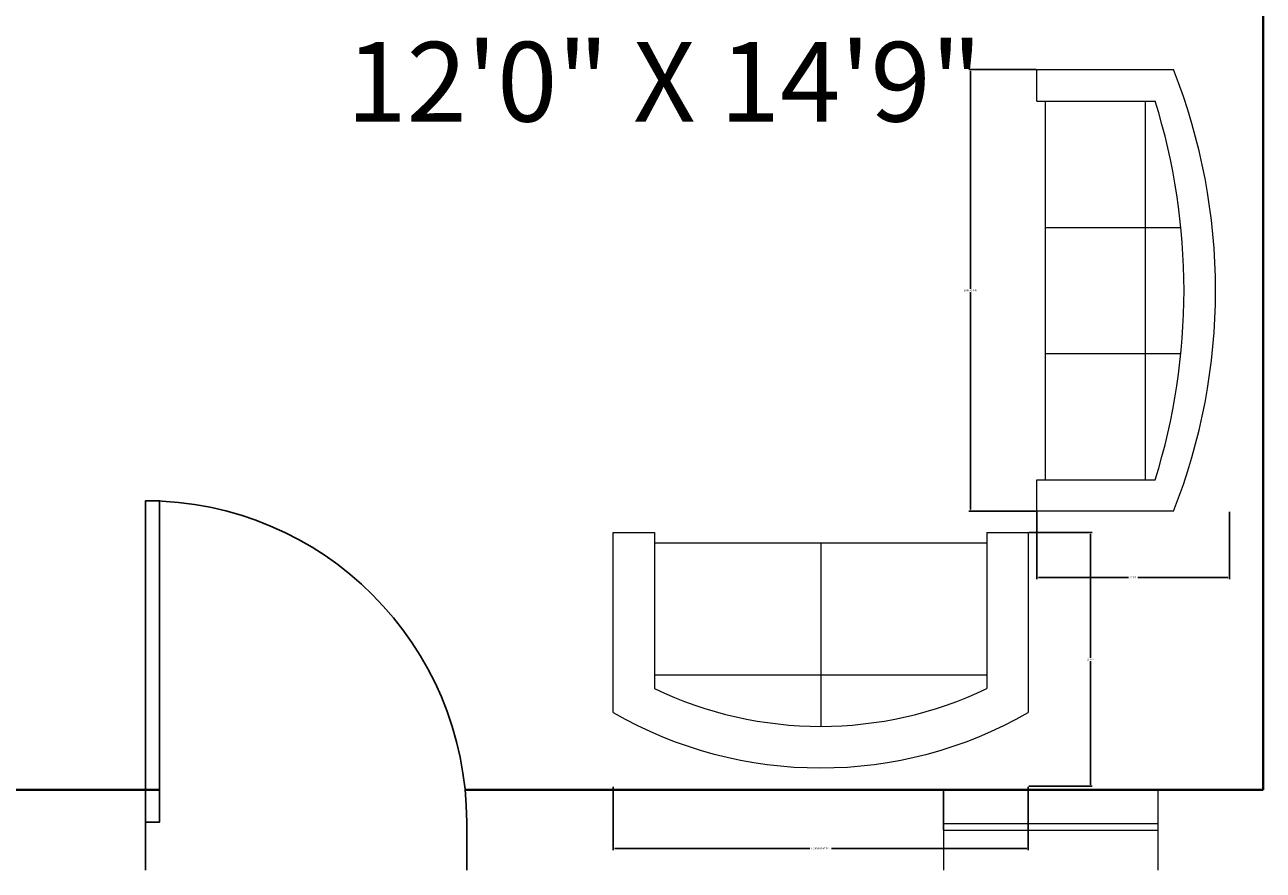
# Model space of a CAD drawing. Units: inches. Extents: x -46 to 1145, y -527 to 760.
# Tile 45 of 57: x 195 to 334, y 222 to 316. Entities that reach past the tile are written whole.
import ezdxf

# ---------------------------------------------------------------- set-up
doc = ezdxf.new("R2010")
doc.units = ezdxf.units.IN
doc.header["$MEASUREMENT"] = 0
for name, color, linetype, lineweight in [('A-ANNO-DIMS', 2, 'Continuous', 18), ('A-AREA-IDEN', 1, 'Continuous', 18), ('A-FURN', 2, 'Continuous', 13), ('DOORS', 3, 'Continuous', 25), ('WALLS', 4, 'Continuous', 40), ('WINDOWS', 240, 'Continuous', 20)]:
    doc.layers.add(name, color=color, linetype=linetype, lineweight=lineweight)
doc.styles.get("Standard").update_dxf_attribs({"font": 'arial.ttf'})
doc.dimstyles.get("Standard").update_dxf_attribs({"dimtxt": 0.18, "dimasz": 0.18, "dimexe": 0.18, "dimexo": 0.0625, "dimgap": 0.09, "dimtad": 0, "dimtih": 1, "dimtoh": 1, "dimdec": 0, "dimzin": 0, "dimdsep": 46, "dimlunit": 3, "dimtxsty": 'Standard', "dimcen": 0.09, "dimadec": 0, "dimazin": 0, "dimtfac": 1, "dimtdec": 0, "dimtofl": 0, "dimtmove": 0, "dimatfit": 3, "dimfxl": 1, "dimtolj": 1, "dimtzin": 0, "dimarcsym": 0})

# ---------------------------------------------------------------- blocks, each defined once
blk = doc.blocks.new('Sofa - Roundback 7 ft.')
for p, q in [((-12.00002, -32.4421), (-12.00003, -6.5971)), ((11.99997, -32.4421), (11.99998, -6.5971)), ((-36.000027, -34), (-36.000027, -11.4696)), ((35.99998, -34), (35.99998, -11.4696)), ((-35.999844, -13.3819), (35.9998, -13.3819)), ((-36.000027, -32.4421), (35.99998, -32.4421))]:
    blk.add_line(p, q)
for points in [[(-36.000027, -34), (-42.000027, -34), (-42.000027, -8)], [(41.99998, -8), (41.99998, -34), (35.99998, -34)]]:
    blk.add_lwpolyline(points)
for centre, radius, start, end in [((0, -114.25), 114.25, 68.43141, 111.5686), ((-0.00001, -127.1968), 121.1968, 72.72033, 107.2797)]:
    blk.add_arc(centre, radius, start, end)
blk = doc.blocks.new('Sofa - Roundback Loveseat 5 ft.')
for p, q in [((0, -32.44198), (0, -5.99998)), ((-24, -33.99998), (-24, -11.46958)), ((24.00004, -33.99998), (24.00004, -11.46958)), ((-23.9998, -13.38178), (23.99986, -13.38178)), ((-24, -32.44198), (24.00004, -32.44198))]:
    blk.add_line(p, q)
for points in [[(-24, -33.99998), (-30, -33.99998), (-30, -7.99998)], [(30.00004, -7.99998), (30.00004, -33.99998), (24.00004, -33.99998)]]:
    blk.add_lwpolyline(points)
for centre, radius, start, end in [((0, -60.24998), 60.24998, 60.13715, 119.8628), ((0, -61.38438), 55.38444, 64.32083, 115.6792)]:
    blk.add_arc(centre, radius, start, end)
blk = doc.blocks.new('*U2')
for p, q in [((0, 0), (0, -6)), ((40, 0), (40, -6))]:
    blk.add_line(p, q)
blk.add_lwpolyline([(0, 0), (0, 40), (1.75, 40), (1.75, 0)], close=True)
blk.add_arc((0, 0), 40, 0, 90)
blk = doc.blocks.new('WINDOW-24IN')
for p, q in [((0, 4.5), (0, 9)), ((0, 9), (0, 0)), ((24, 9), (24, 0)), ((0, 5.23), (24, 5.23)), ((0, 4.5), (24, 4.5))]:
    blk.add_line(p, q)
blk = doc.blocks.new('*D670')
at = {"layer": 'A-ANNO-DIMS', "color": 0, "lineweight": -2, "transparency": 16777216}
for p, q in [((308.12, 311.23), (300.58, 311.23)), ((300.76, 311.05), (300.76, 286.67)), ((300.76, 261.92), (300.76, 286.3)), ((308.12, 261.74), (300.58, 261.74))]:
    blk.add_line(p, q, dxfattribs=at)
at = {"layer": 'A-ANNO-DIMS', "color": 0, "transparency": 16777216}
for points in [[(300.73, 311.05), (300.79, 311.05), (300.76, 311.23)], [(300.73, 261.92), (300.79, 261.92), (300.76, 261.74)]]:
    blk.add_solid(points, dxfattribs=at)
at = {"layer": 'Defpoints', "color": 0, "transparency": 16777216}
for p in [(308.18, 311.23), (300.76, 261.74), (308.18, 261.74)]:
    blk.add_point(p, dxfattribs=at)
at = {"layer": 'A-ANNO-DIMS', "color": 0, "transparency": 16777216, "insert": (300.76, 286.48), "char_height": 0.18, "attachment_point": 5}
blk.add_mtext('\\A1;SOFA 49 TYP.', dxfattribs=at)
blk = doc.blocks.new('*D671')
at = {"layer": 'A-ANNO-DIMS', "color": 0, "lineweight": -2, "transparency": 16777216}
for p, q in [((308.18, 261.67), (308.18, 254.13)), ((329.79, 261.67), (329.79, 254.13)), ((308.36, 254.31), (318.46, 254.31)), ((329.61, 254.31), (319.52, 254.31))]:
    blk.add_line(p, q, dxfattribs=at)
at = {"layer": 'A-ANNO-DIMS', "color": 0, "transparency": 16777216}
for points in [[(308.36, 254.34), (308.36, 254.28), (308.18, 254.31)], [(329.61, 254.34), (329.61, 254.28), (329.79, 254.31)]]:
    blk.add_solid(points, dxfattribs=at)
at = {"layer": 'Defpoints', "color": 0, "transparency": 16777216}
for p in [(308.18, 261.74), (329.79, 261.74), (329.79, 254.31)]:
    blk.add_point(p, dxfattribs=at)
at = {"layer": 'A-ANNO-DIMS', "color": 0, "transparency": 16777216, "insert": (318.99, 254.31), "char_height": 0.18, "attachment_point": 5}
blk.add_mtext('\\A1;22 TYP.', dxfattribs=at)
blk = doc.blocks.new('*D678')
at = {"layer": 'A-ANNO-DIMS', "color": 0, "lineweight": -2, "transparency": 16777216}
for p, q in [((260.69, 230.86), (260.69, 223.76)), ((307.23, 230.86), (307.23, 223.76)), ((260.87, 223.94), (282.73, 223.94)), ((307.05, 223.94), (285.18, 223.94))]:
    blk.add_line(p, q, dxfattribs=at)
at = {"layer": 'A-ANNO-DIMS', "color": 0, "transparency": 16777216}
for points in [[(260.87, 223.97), (260.87, 223.91), (260.69, 223.94)], [(307.05, 223.97), (307.05, 223.91), (307.23, 223.94)]]:
    blk.add_solid(points, dxfattribs=at)
at = {"layer": 'Defpoints', "color": 0, "transparency": 16777216}
for p in [(260.69, 230.92), (307.23, 230.92), (260.69, 223.94)]:
    blk.add_point(p, dxfattribs=at)
at = {"layer": 'A-ANNO-DIMS', "color": 0, "transparency": 16777216, "insert": (283.96, 223.94), "char_height": 0.18, "attachment_point": 5}
blk.add_mtext('\\A1;LOVESEAT 47 TYP.', dxfattribs=at)
blk = doc.blocks.new('*D679')
at = {"layer": 'A-ANNO-DIMS', "color": 0, "lineweight": -2, "transparency": 16777216}
for p, q in [((307.29, 259.36), (314.39, 259.36)), ((314.21, 259.18), (314.21, 245.32)), ((314.21, 231.1), (314.21, 244.96)), ((307.29, 230.92), (314.39, 230.92))]:
    blk.add_line(p, q, dxfattribs=at)
at = {"layer": 'A-ANNO-DIMS', "color": 0, "transparency": 16777216}
for points in [[(314.18, 259.18), (314.24, 259.18), (314.21, 259.36)], [(314.18, 231.1), (314.24, 231.1), (314.21, 230.92)]]:
    blk.add_solid(points, dxfattribs=at)
at = {"layer": 'Defpoints', "color": 0, "transparency": 16777216}
for p in [(307.23, 259.36), (307.23, 230.92), (314.21, 230.92)]:
    blk.add_point(p, dxfattribs=at)
at = {"layer": 'A-ANNO-DIMS', "color": 0, "transparency": 16777216, "insert": (314.21, 245.14), "char_height": 0.18, "attachment_point": 5}
blk.add_mtext('\\A1;28 TYP.', dxfattribs=at)

msp = doc.modelspace()

# ---------------------------------------------------------------- linework, layer by layer
at = {"layer": 'WALLS'}
for p, q in [((333.5637, 331.232), (333.5637, 230.5176)), ((209.8481, 230.5176), (189.5637, 230.5176)), ((333.5637, 230.5176), (244.0926, 230.5176))]:
    msp.add_line(p, q, dxfattribs=at)

# ---------------------------------------------------------------- block references
at = {"layer": 'A-FURN'}
for name, p, xscale, yscale, zscale, rotation in [('Sofa - Roundback 7 ft.', (328.2179, 286.4838), 0.5892128430585409, 0.5892128430585409, 0.5892128430585409, 270), ('Sofa - Roundback Loveseat 5 ft.', (283.9562, 232.9861), 0.7756934806711657, 0.7756934806711657, 0.7756934806711657, 180)]:
    msp.add_blockref(name, p, dxfattribs=dict(at, xscale=xscale, yscale=yscale, zscale=zscale, rotation=rotation))
at = {"layer": 'DOORS', "xscale": 0.9, "yscale": 0.9, "zscale": 0.9}
msp.add_blockref('*U2', (208.2731, 226.9176), dxfattribs=at)
at = {"layer": 'WINDOWS'}
msp.add_blockref('WINDOW-24IN', (297.733, 221.518), dxfattribs=at)

# ---------------------------------------------------------------- texts
at = {"layer": 'A-AREA-IDEN'}
msp.add_text('12\'0" X 14\'9"', height=8.923264, dxfattribs=at).set_placement((230.7854, 305.4112))

# ---------------------------------------------------------------- dimensions: what is measured, and where the dimension line sits
at = {"layer": 'A-ANNO-DIMS'}
for base, p1, p2, angle, text, picture, middle in [((300.7606, 261.7369), (308.1846, 311.2307), (308.1846, 261.7369), 270, 'SOFA <> TYP.', '*D670', (300.7606, 286.4838)), ((314.2083, 230.9176), (307.227, 259.3597), (307.227, 230.9176), 270, '<> TYP.', '*D679', (314.2083, 245.1386)), ((260.6854, 223.9363), (307.227, 230.9176), (260.6854, 230.9176), 180, 'LOVESEAT <> TYP.', '*D678', (283.9562, 223.9363))]:
    dim = msp.add_linear_dim(base=base, p1=p1, p2=p2, angle=angle, text=text, dimstyle='Standard', override={"dimdec": 0, "dimlfac": 1, "dimrnd": 0, "dimzin": 0, "dimdsep": 46, "dimlunit": 2}, dxfattribs=at)
    dim.commit()
    dim.dimension.update_dxf_attribs({"geometry": picture, "text_midpoint": middle})
dim = msp.add_linear_dim(base=(329.7891, 254.3128), p1=(308.1846, 261.7369), p2=(329.7891, 261.7369), text='<> TYP.', dimstyle='Standard', override={"dimdec": 0, "dimlfac": 1, "dimrnd": 0, "dimzin": 0, "dimdsep": 46, "dimlunit": 2}, dxfattribs=at)
dim.commit()
dim.dimension.update_dxf_attribs({"geometry": '*D671', "text_midpoint": (318.9869, 254.3128)})

doc.saveas('drawing.dxf')
